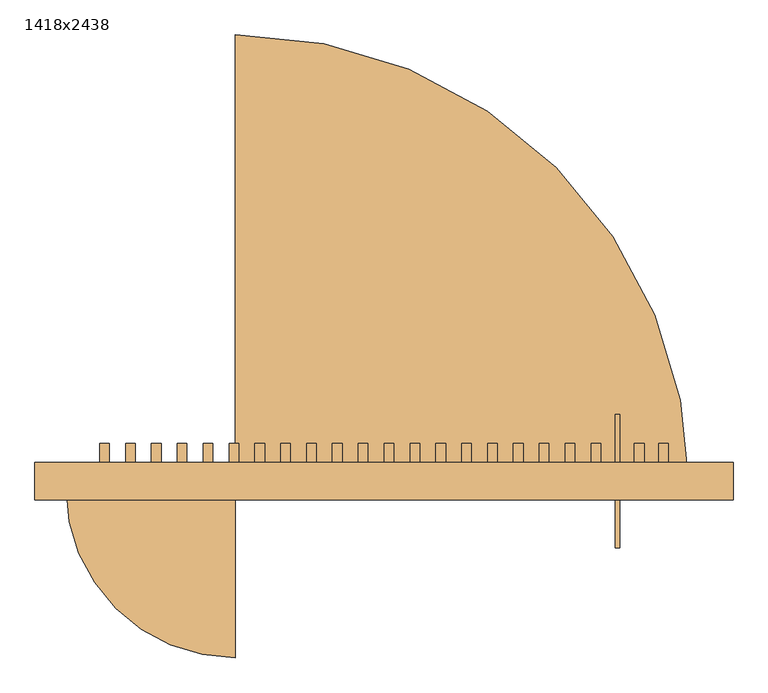
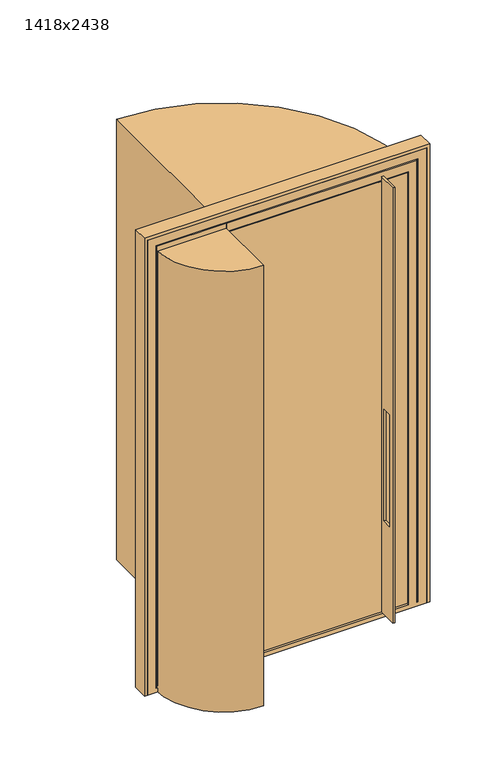
"""IFC4 building model written with IfcOpenShell, lengths in millimetres: door geometry, 1418x2438."""

from ifc_helpers import new_model, si_unit, point, frame, frame_2d, origin, origin_with_axes, place, context, project, spatial, polyline, circle_curve, trimmed, segment, composite_curve, outline, extrude, faceted_brep, source, transform, mapped, element, save


def door_1418x2438_e3a65d4f(model_context):
    return source(origin(), model_context, "Body", "SolidModel", [
        extrude(outline(composite_curve([segment(polyline([(-308.75, 40.3), (-308.75, -310.2)]), True, "CONTINUOUS"), segment(trimmed(circle_curve(frame_2d((-308.75, 40.3)), 350.5), [point((-308.75, -310.2))], [point((-659.25, 40.3))], False, "CARTESIAN"), True, "CONTINUOUS"), segment(polyline([(-659.25, 40.3), (-308.75, 40.3)]), True, "CONTINUOUS")], self_intersect=False)), origin_with_axes(), (0.0, 0.0, 1.0), 2362.4),
        extrude(outline(composite_curve([segment(polyline([(-308.75, 40.3), (-308.75, 981.8)]), True, "CONTINUOUS"), segment(trimmed(circle_curve(frame_2d((-308.75, 40.3)), 941.5), [point((-308.75, 981.8))], [point((632.75, 40.3))], False, "CARTESIAN"), True, "CONTINUOUS"), segment(polyline([(632.75, 40.3), (-308.75, 40.3)]), True, "CONTINUOUS")], self_intersect=False)), origin_with_axes(), (0.0, 0.0, 1.0), 2362.4),
        extrude(outline(polyline([(194.3, 2363.9), (194.3, 30.0), (94.3, 30.0), (94.3, 2363.9), (194.3, 2363.9)]), holes=[polyline([(164.3, 1130.0), (114.3, 1130.0), (114.3, 530.0), (164.3, 530.0), (164.3, 1130.0)])]), frame((479.25, 0.0, 0.0), z_axis=(1.0, 0.0, 0.0), x_axis=(0.0, 1.0, 0.0)), (0.0, 0.0, 1.0), 10.0),
        extrude(outline(polyline([(-82.7, 2363.9), (17.3, 2363.9), (17.3, 30.0), (-82.7, 30.0), (-82.7, 2363.9)]), holes=[polyline([(-52.7, 1130.0), (-52.7, 530.0), (-2.7, 530.0), (-2.7, 1130.0), (-52.7, 1130.0)])]), frame((479.25, 0.0, 0.0), z_axis=(1.0, 0.0, 0.0), x_axis=(0.0, 1.0, 0.0)), (0.0, 0.0, 1.0), 10.0),
        extrude(outline(polyline([(375.6447368, 134.3), (395.6447368, 134.3), (395.6447368, 94.3), (375.6447368, 94.3), (375.6447368, 134.3)])), frame((0.0, 0.0, 30.0), z_axis=(0.0, 0.0, 1.0), x_axis=(1.0, 0.0, 0.0)), (0.0, 0.0, 1.0), 2333.9),
        extrude(outline(polyline([(322.0394737, 134.3), (342.0394737, 134.3), (342.0394737, 94.3), (322.0394737, 94.3), (322.0394737, 134.3)])), frame((0.0, 0.0, 30.0), z_axis=(0.0, 0.0, 1.0), x_axis=(1.0, 0.0, 0.0)), (0.0, 0.0, 1.0), 2333.9),
        extrude(outline(polyline([(268.4342105, 134.3), (288.4342105, 134.3), (288.4342105, 94.3), (268.4342105, 94.3), (268.4342105, 134.3)])), frame((0.0, 0.0, 30.0), z_axis=(0.0, 0.0, 1.0), x_axis=(1.0, 0.0, 0.0)), (0.0, 0.0, 1.0), 2333.9),
        extrude(outline(polyline([(214.8289474, 134.3), (234.8289474, 134.3), (234.8289474, 94.3), (214.8289474, 94.3), (214.8289474, 134.3)])), frame((0.0, 0.0, 30.0), z_axis=(0.0, 0.0, 1.0), x_axis=(1.0, 0.0, 0.0)), (0.0, 0.0, 1.0), 2333.9),
        extrude(outline(polyline([(161.2236842, 134.3), (181.2236842, 134.3), (181.2236842, 94.3), (161.2236842, 94.3), (161.2236842, 134.3)])), frame((0.0, 0.0, 30.0), z_axis=(0.0, 0.0, 1.0), x_axis=(1.0, 0.0, 0.0)), (0.0, 0.0, 1.0), 2333.9),
        extrude(outline(polyline([(107.6184211, 134.3), (127.6184211, 134.3), (127.6184211, 94.3), (107.6184211, 94.3), (107.6184211, 134.3)])), frame((0.0, 0.0, 30.0), z_axis=(0.0, 0.0, 1.0), x_axis=(1.0, 0.0, 0.0)), (0.0, 0.0, 1.0), 2333.9),
        extrude(outline(polyline([(54.0131579, 134.3), (74.0131579, 134.3), (74.0131579, 94.3), (54.0131579, 94.3), (54.0131579, 134.3)])), frame((0.0, 0.0, 30.0), z_axis=(0.0, 0.0, 1.0), x_axis=(1.0, 0.0, 0.0)), (0.0, 0.0, 1.0), 2333.9),
        extrude(outline(polyline([(0.4078947, 134.3), (20.4078947, 134.3), (20.4078947, 94.3), (0.4078947, 94.3), (0.4078947, 134.3)])), frame((0.0, 0.0, 30.0), z_axis=(0.0, 0.0, 1.0), x_axis=(1.0, 0.0, 0.0)), (0.0, 0.0, 1.0), 2333.9),
        extrude(outline(polyline([(-53.1973684, 134.3), (-33.1973684, 134.3), (-33.1973684, 94.3), (-53.1973684, 94.3), (-53.1973684, 134.3)])), frame((0.0, 0.0, 30.0), z_axis=(0.0, 0.0, 1.0), x_axis=(1.0, 0.0, 0.0)), (0.0, 0.0, 1.0), 2333.9),
        extrude(outline(polyline([(-106.8026316, 134.3), (-86.8026316, 134.3), (-86.8026316, 94.3), (-106.8026316, 94.3), (-106.8026316, 134.3)])), frame((0.0, 0.0, 30.0), z_axis=(0.0, 0.0, 1.0), x_axis=(1.0, 0.0, 0.0)), (0.0, 0.0, 1.0), 2333.9),
        extrude(outline(polyline([(-160.4078947, 134.3), (-140.4078947, 134.3), (-140.4078947, 94.3), (-160.4078947, 94.3), (-160.4078947, 134.3)])), frame((0.0, 0.0, 30.0), z_axis=(0.0, 0.0, 1.0), x_axis=(1.0, 0.0, 0.0)), (0.0, 0.0, 1.0), 2333.9),
        extrude(outline(polyline([(-214.0131579, 134.3), (-194.0131579, 134.3), (-194.0131579, 94.3), (-214.0131579, 94.3), (-214.0131579, 134.3)])), frame((0.0, 0.0, 30.0), z_axis=(0.0, 0.0, 1.0), x_axis=(1.0, 0.0, 0.0)), (0.0, 0.0, 1.0), 2333.9),
        extrude(outline(polyline([(-267.6184211, 134.3), (-247.6184211, 134.3), (-247.6184211, 94.3), (-267.6184211, 94.3), (-267.6184211, 134.3)])), frame((0.0, 0.0, 30.0), z_axis=(0.0, 0.0, 1.0), x_axis=(1.0, 0.0, 0.0)), (0.0, 0.0, 1.0), 2333.9),
        extrude(outline(polyline([(-321.2236842, 134.3), (-301.2236842, 134.3), (-301.2236842, 94.3), (-321.2236842, 94.3), (-321.2236842, 134.3)])), frame((0.0, 0.0, 30.0), z_axis=(0.0, 0.0, 1.0), x_axis=(1.0, 0.0, 0.0)), (0.0, 0.0, 1.0), 2333.9),
        extrude(outline(polyline([(-374.8289474, 134.3), (-354.8289474, 134.3), (-354.8289474, 94.3), (-374.8289474, 94.3), (-374.8289474, 134.3)])), frame((0.0, 0.0, 30.0), z_axis=(0.0, 0.0, 1.0), x_axis=(1.0, 0.0, 0.0)), (0.0, 0.0, 1.0), 2333.9),
        extrude(outline(polyline([(-428.4342105, 134.3), (-408.4342105, 134.3), (-408.4342105, 94.3), (-428.4342105, 94.3), (-428.4342105, 134.3)])), frame((0.0, 0.0, 30.0), z_axis=(0.0, 0.0, 1.0), x_axis=(1.0, 0.0, 0.0)), (0.0, 0.0, 1.0), 2333.9),
        extrude(outline(polyline([(-482.0394737, 134.3), (-462.0394737, 134.3), (-462.0394737, 94.3), (-482.0394737, 94.3), (-482.0394737, 134.3)])), frame((0.0, 0.0, 30.0), z_axis=(0.0, 0.0, 1.0), x_axis=(1.0, 0.0, 0.0)), (0.0, 0.0, 1.0), 2333.9),
        extrude(outline(polyline([(-535.6447368, 134.3), (-515.6447368, 134.3), (-515.6447368, 94.3), (-535.6447368, 94.3), (-535.6447368, 134.3)])), frame((0.0, 0.0, 30.0), z_axis=(0.0, 0.0, 1.0), x_axis=(1.0, 0.0, 0.0)), (0.0, 0.0, 1.0), 2333.9),
        extrude(outline(polyline([(429.25, 134.3), (449.25, 134.3), (449.25, 94.3), (429.25, 94.3), (429.25, 134.3)])), frame((0.0, 0.0, 30.0), z_axis=(0.0, 0.0, 1.0), x_axis=(1.0, 0.0, 0.0)), (0.0, 0.0, 1.0), 2333.9),
        extrude(outline(polyline([(-589.25, 134.3), (-569.25, 134.3), (-569.25, 94.3), (-589.25, 94.3), (-589.25, 134.3)])), frame((0.0, 0.0, 30.0), z_axis=(0.0, 0.0, 1.0), x_axis=(1.0, 0.0, 0.0)), (0.0, 0.0, 1.0), 2333.9),
        extrude(outline(polyline([(429.25, 134.3), (449.25, 134.3), (449.25, 94.3), (429.25, 94.3), (429.25, 134.3)])), frame((0.0, 0.0, 30.0), z_axis=(0.0, 0.0, 1.0), x_axis=(1.0, 0.0, 0.0)), (0.0, 0.0, 1.0), 2333.9),
        extrude(outline(polyline([(519.25, 134.3), (539.25, 134.3), (539.25, 94.3), (519.25, 94.3), (519.25, 134.3)])), frame((0.0, 0.0, 30.0), z_axis=(0.0, 0.0, 1.0), x_axis=(1.0, 0.0, 0.0)), (0.0, 0.0, 1.0), 2333.9),
        extrude(outline(polyline([(569.25, 134.3), (589.25, 134.3), (589.25, 94.3), (569.25, 94.3), (569.25, 134.3)])), frame((0.0, 0.0, 30.0), z_axis=(0.0, 0.0, 1.0), x_axis=(1.0, 0.0, 0.0)), (0.0, 0.0, 1.0), 2333.9),
        extrude(outline(polyline([(78.7737686, 20.0), (63.8262314, 20.0), (61.9659828, 22.3999036), (60.9985837, 24.7725969), (81.6014163, 24.7725969), (80.6340172, 22.3999036), (78.7737686, 20.0)])), frame((-609.25, 0.0, 0.0), z_axis=(1.0, 0.0, 0.0), x_axis=(0.0, 1.0, 0.0)), (0.0, 0.0, 1.0), 1218.5),
        faceted_brep([(-634.25, 94.3, 2363.9), (-634.25, 94.3, 30.0), (-634.25, 85.3, 30.0), (-634.25, 85.3, 2363.9), (-308.75, 85.3, 2363.9), (-308.75, 85.3, 2370.4), (-308.75, 26.3, 2370.4), (-308.75, 26.3, 2388.9), (-308.75, 17.3, 2388.9), (-308.75, 17.3, 2343.9), (-308.75, 26.3, 2343.9), (-308.75, 26.3, 2345.4), (-308.75, 85.3, 2345.4), (634.25, 85.3, 2363.9), (634.25, 94.3, 2363.9), (-609.25, 27.45, 30.0), (-609.25, 27.45, 28.5), (609.25, 27.45, 28.5), (609.25, 27.45, 30.0), (-609.25, 81.700043, 24.7725969), (-609.25, 81.700043, 30.0), (609.25, 81.700043, 30.0), (609.25, 81.700043, 24.7725969), (-609.25, 60.899957, 24.7725969), (-609.25, 60.899957, 28.5), (-609.25, 17.3, 2338.9), (-609.25, 26.3, 2338.9), (-609.25, 26.3, 30.0), (-609.25, 17.3, 30.0), (609.25, 60.899957, 28.5), (609.25, 60.899957, 24.7725969), (609.25, 26.3, 2338.9), (609.25, 17.3, 2338.9), (609.25, 17.3, 30.0), (609.25, 26.3, 30.0), (634.25, 94.3, 30.0), (634.25, 85.3, 30.0), (615.75, 85.3, 30.0), (615.75, 26.3, 30.0), (-614.25, 26.3, 30.0), (-614.25, 17.3, 30.0), (-659.25, 17.3, 30.0), (-659.25, 26.3, 30.0), (-640.75, 26.3, 30.0), (-640.75, 85.3, 30.0), (-640.75, 85.3, 2370.4), (615.75, 85.3, 2345.4), (615.75, 26.3, 2345.4), (-659.25, 17.3, 2388.9), (-659.25, 26.3, 2388.9), (-640.75, 26.3, 2370.4), (-614.25, 26.3, 2343.9), (-614.25, 17.3, 2343.9)], [[[0, 1, 2, 3]], [[4, 5, 6, 7, 8, 9, 10, 11, 12]], [[0, 3, 4, 13, 14]], [[15, 16, 17, 18]], [[19, 20, 21, 22]], [[20, 19, 23, 24, 16, 15]], [[25, 26, 27, 28]], [[16, 24, 29, 17]], [[24, 23, 30, 29]], [[18, 17, 29, 30, 22, 21]], [[31, 32, 33, 34]], [[1, 0, 14, 35]], [[2, 1, 35, 36, 37, 38, 34, 33, 28, 27, 39, 40, 41, 42, 43, 44], [20, 15, 18, 21]], [[25, 28, 33, 32]], [[36, 35, 14, 13]], [[5, 4, 3, 2, 44, 45]], [[38, 37, 46, 47]], [[42, 41, 48, 49]], [[7, 6, 50, 43, 42, 49]], [[44, 43, 50, 45]], [[37, 36, 13, 4, 12, 46]], [[11, 47, 46, 12]], [[6, 5, 45, 50]], [[8, 7, 49, 48]], [[39, 27, 26, 31, 34, 38, 47, 11, 10, 51]], [[40, 39, 51, 52]], [[9, 8, 48, 41, 40, 52]], [[10, 9, 52, 51]], [[26, 25, 32, 31]], [[23, 19, 22, 30]]]),
        extrude(outline(polyline([(0.0, 708.75), (0.0, 723.75), (2453.4, 723.75), (2453.4, -723.75), (0.0, -723.75), (0.0, -708.75), (2438.4, -708.75), (2438.4, 708.75), (0.0, 708.75)])), frame((0.0, 17.3, 0.0), z_axis=(0.0, 1.0, 0.0), x_axis=(0.0, 0.0, 1.0)), (0.0, 0.0, 1.0), 77.0),
        faceted_brep([(-708.75, 94.3, 0.0), (-708.75, 17.3, 0.0), (-708.75, 17.3, 2438.4), (-708.75, 94.3, 2438.4), (708.75, 17.3, 0.0), (708.75, 94.3, 0.0), (708.75, 94.3, 2438.4), (708.75, 17.3, 2438.4), (664.25, 17.3, 2393.9), (664.25, 17.3, 20.0), (659.25, 17.3, 20.0), (659.25, 17.3, 2388.9), (-308.75, 17.3, 2388.9), (-308.75, 17.3, 2343.9), (614.25, 17.3, 2343.9), (614.25, 17.3, 20.0), (-664.25, 17.3, 20.0), (-664.25, 17.3, 2393.9), (-639.25, 94.3, 20.0), (639.25, 94.3, 20.0), (639.25, 94.3, 2368.9), (-639.25, 94.3, 2368.9), (-639.25, 85.3, 2368.9), (-639.25, 85.3, 20.0), (639.25, 85.3, 2368.9), (-308.75, 85.3, 2368.9), (-308.75, 85.3, 2387.4), (-657.75, 85.3, 2387.4), (-657.75, 85.3, 20.0), (-657.75, 26.3, 2387.4), (-657.75, 26.3, 20.0), (-308.75, 26.3, 2387.4), (-308.75, 26.3, 2388.9), (659.25, 26.3, 2388.9), (659.25, 26.3, 20.0), (664.25, 26.3, 20.0), (664.25, 26.3, 2393.9), (-664.25, 26.3, 2393.9), (-664.25, 26.3, 20.0), (614.25, 26.3, 20.0), (632.75, 26.3, 20.0), (632.75, 85.3, 20.0), (639.25, 85.3, 20.0), (-308.75, 85.3, 2362.4), (-308.75, 26.3, 2362.4), (-308.75, 26.3, 2343.9), (632.75, 85.3, 2362.4), (632.75, 26.3, 2362.4), (614.25, 26.3, 2343.9)], [[[0, 1, 2, 3]], [[4, 5, 6, 7]], [[4, 7, 2, 1], [8, 9, 10, 11, 12, 13, 14, 15, 16, 17]], [[6, 5, 0, 3], [18, 19, 20, 21]], [[4, 1, 0, 5]], [[21, 22, 23, 18]], [[6, 3, 2, 7]], [[22, 21, 20, 24, 25]], [[23, 22, 25, 26, 27, 28]], [[27, 29, 30, 28]], [[30, 29, 31, 32, 33, 34, 35, 36, 37, 38]], [[37, 17, 16, 38]], [[29, 27, 26, 31]], [[8, 17, 37, 36]], [[10, 9, 35, 34]], [[18, 23, 28, 30, 38, 16, 15, 39, 40, 41, 42, 19]], [[25, 43, 44, 45, 13, 12, 32, 31, 26]], [[43, 25, 24, 42, 41, 46]], [[44, 43, 46, 47]], [[45, 44, 47, 40, 39, 48]], [[13, 45, 48, 14]], [[33, 32, 12, 11]], [[24, 20, 19, 42]], [[47, 46, 41, 40]], [[14, 48, 39, 15]], [[33, 11, 10, 34]], [[8, 36, 35, 9]]]),
    ])


if __name__ == "__main__":
    model = new_model("IFC4")
    model_context = context("Model", 3, world=origin())
    ifc_project = project(units=[si_unit("LENGTHUNIT", "METRE", prefix="MILLI")], contexts=[model_context])
    site = spatial("IfcSite", under=ifc_project)
    building = spatial("IfcBuilding", under=site)
    placement = place(None, origin())
    door_1418x2438_shape = door_1418x2438_e3a65d4f(model_context)
    element("IfcDoor", 1, ObjectType="1418x2438", at=placement, inside=building, context=model_context, shape_type="MappedRepresentation", body=[
        mapped(door_1418x2438_shape, transform((0.0, 0.0, 0.0), x_axis=(1.0, 0.0, 0.0), y_axis=(0.0, 1.0, 0.0), z_axis=(0.0, 0.0, 1.0))),
    ])
    save(model, "model.ifc")

# Revit data of these elements
# Type "1418x2438"
#   Type Mark = "8"
#   Type IFC Predefined Type = "USERDEFINED"
#   Export Type to IFC As = "IfcDoorType"
#   Water resistance = "up to Class 3B, EN 12208"
#   URL = "https://aluprof.com/en/architects/contact/contact-bim"
#   Right-hand / Left-hand door [instance default] = ""
#   Resistance to wind load = "up to Class C3, EN 12210"
#   Operation = "SinglePanelOutwardOpening"
#   Opening type = "Outward"
#   Model = "MB-86N Pivot Door"
#   ManufacturerSustainabilityPolicyURL [instance default] = "https://aluprof.com/en/company/sustainable-development"
#   Manufacturer = "ALUPROF SA"
#   Keynote = "08131600"
#   Insert type = "SI+"
#   IfcExportType = "USERDEFINED"
#   IfcExportAs = "IfcDoorType"
#   Hardware [instance default] = "Wala"
#   Handle type [instance default] = "Exterior: Handrail, Interior: Handrail"
#   Glazing construction = ""
#   Door sill type [instance default] = ""
#   Description = "External single door outward opening"
#   Content of the recyclate in the material = "69.2%"
#   COBie.Type.Name = "MB-86N"
#   COBie.Type.Manufacturer = "ALUPROF SA"
#   Assembly Code = "B2030110"
#   Analytic Construction = "<None>"
#   Air permeability = "up to Class 3, EN 12207"
#   Base rotation offset = 1' - 3.74803"
#   Thickness = 0' - 3.0315"
#   Thermal insulation = 0.153216 BTU/(h·ft²·°F)
#   Rough Width = 4' - 8.98819"
#   Rough Height = 4' - 8.39764"
#   Rotation angle [instance default] = 0.00°
#   Rotation Offset = 1' - 3.74803"
#   Mounting space bottom = 0' - 0"
#   Mounting space = 0' - 0.59055"
#   Frame Width = 0' - 3.0315"
#   Height = 8' - 0"
#   Width = 4' - 7.80709"
#   Floor finish level [instance default] = 0' - 0"
#   Exterior wall face offset = 0' - 0.7874"
#   Clear opening width = 2' - 11.43307"
#   Clear opening height = 7' - 7.49213"
#   Handrail [instance default] = yes
#   Thermal variant SI+ = yes
#   ShowClearanceZone [instance default] = yes
#   Schedule No. = 1
#   IsExternal = yes
#   IsDoorOpen [instance default] = no
#   IsDoorClosed [instance default] = yes
#   Handrail - Handrail [instance default] = yes
#   Function = 1
#   Door closer [instance default] = yes
#   Define Thermal Properties by = 1
#   COBie.Type = yes
#   COBie = yes
#   Access control [instance default] = yes
#   Wall Closure = (empty or 0)
# Element 1 (IfcDoor, "1418x2438")
#   Materials on its faces: "Clearance Zone"
# Materials
#   "Clearance Zone": class "Generic", colour RGB 180 0 0, transparency 0.85, Cost = 0
